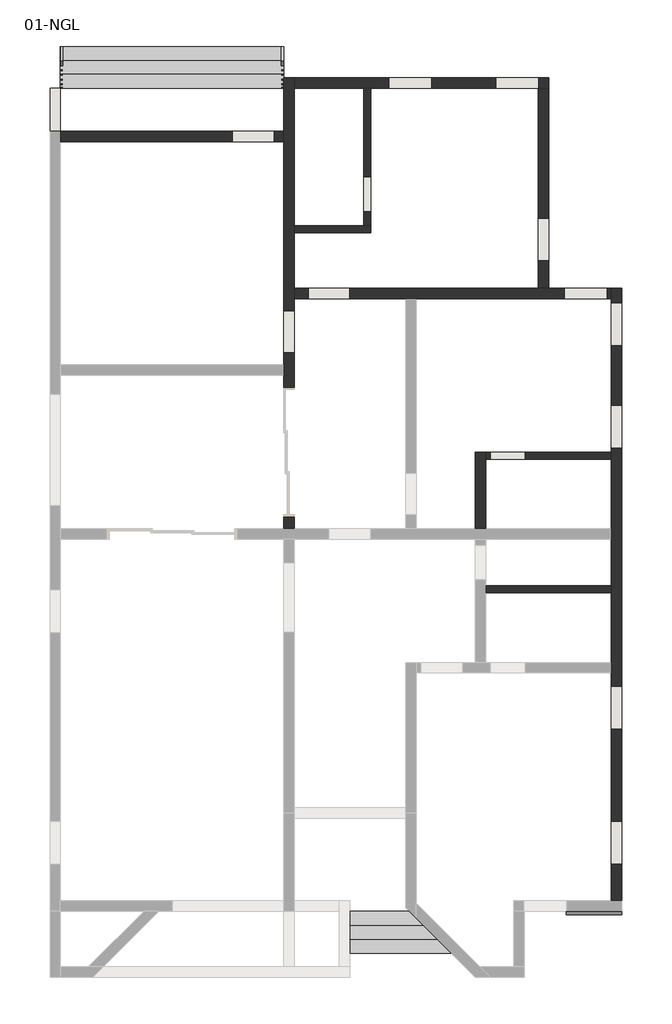
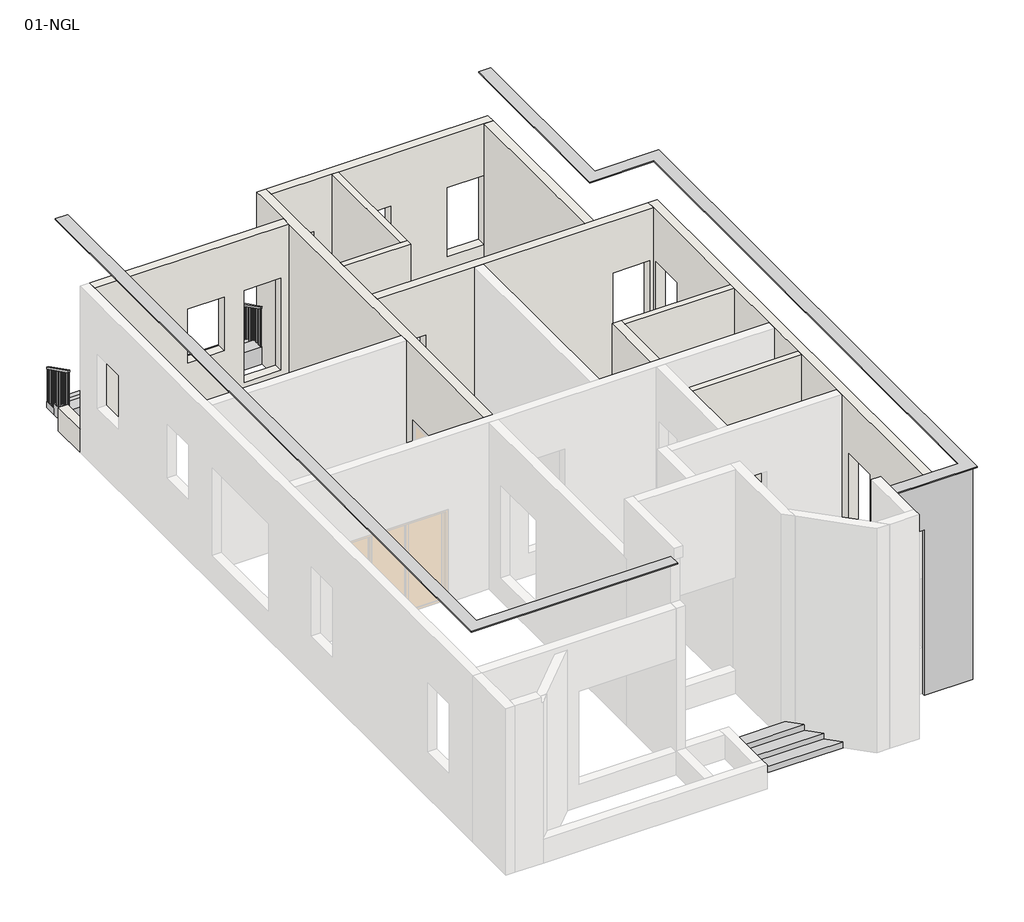
# One storey, part 2 of 2: 12 walls, 2 railings, 2 stair flights, 1 furniture element.
"""IFC4 building model written with IfcOpenShell, lengths in millimetres."""

from ifc_helpers import new_model, si_unit, frame, origin, origin_with_axes, place, context, project, spatial, polyline, outline, extrude, faceted_brep, transform, mapped, element, save
from components import casework_1_casework_1_d55a6497

model = new_model("IFC4")

# Units and contexts
model_context = context("Model", 3, world=origin())
ifc_project = project(units=[si_unit("LENGTHUNIT", "METRE", prefix="MILLI")], contexts=[model_context])

# Site, building, storey
site = spatial("IfcSite", under=ifc_project)
building = spatial("IfcBuilding", under=site)
storey = spatial("IfcBuildingStorey", under=building, Name="01-NGL", Elevation=0.0)

# Furniture
placement = place(None, origin())
casework_1_casework_1_shape = casework_1_casework_1_d55a6497(model_context)
element("IfcFurniture", 1, ObjectType="Casework 1 : Casework 1", at=placement, inside=storey, context=model_context, shape_type="MappedRepresentation", body=[
    mapped(casework_1_casework_1_shape, transform((0.0, 0.0, 0.0), x_axis=(1.0, 0.0, 0.0), y_axis=(0.0, 1.0, 0.0), z_axis=(0.0, 0.0, 1.0))),
])

# Railings
element("IfcRailing", 2, ObjectType="Handrail - Rectangular", at=placement, inside=storey, context=model_context, shape_type="SweptSolid", body=[
    extrude(outline(polyline([(5977.4735, 1050.0), (5977.4735, 994.0983006), (5077.4735, 1444.0983006), (5077.4735, 1500.0), (5977.4735, 1050.0)])), frame((-8660.0564803, 0.0, 0.0), z_axis=(1.0, 0.0, 0.0), x_axis=(0.0, 1.0, 0.0)), (0.0, 0.0, 1.0), 50.0),
    extrude(outline(polyline([(5174.6735, 1395.4983006), (5174.6735, 450.0), (5154.6735, 450.0), (5154.6735, 1405.4983006), (5174.6735, 1395.4983006)])), frame((-8645.0564803, 0.0, 0.0), z_axis=(1.0, 0.0, 0.0), x_axis=(0.0, 1.0, 0.0)), (0.0, 0.0, 1.0), 20.0),
    extrude(outline(polyline([(5276.2735, 1344.6983006), (5276.2735, 450.0), (5256.2735, 450.0), (5256.2735, 1354.6983006), (5276.2735, 1344.6983006)])), frame((-8645.0564803, 0.0, 0.0), z_axis=(1.0, 0.0, 0.0), x_axis=(0.0, 1.0, 0.0)), (0.0, 0.0, 1.0), 20.0),
    extrude(outline(polyline([(5377.8735, 1293.8483006), (5377.8735, 450.0), (5357.8735, 450.0), (5357.8735, 1303.8483006), (5377.8735, 1293.8483006)])), frame((-8645.0564803, 0.0, 0.0), z_axis=(1.0, 0.0, 0.0), x_axis=(0.0, 1.0, 0.0)), (0.0, 0.0, 1.0), 20.0),
    extrude(outline(polyline([(5479.4735, 1243.0983006), (5479.4735, 300.0), (5459.4735, 300.0), (5459.4735, 1253.0983006), (5479.4735, 1243.0983006)])), frame((-8645.0564803, 0.0, 0.0), z_axis=(1.0, 0.0, 0.0), x_axis=(0.0, 1.0, 0.0)), (0.0, 0.0, 1.0), 20.0),
    extrude(outline(polyline([(5581.0735, 1192.2983006), (5581.0735, 300.0), (5561.0735, 300.0), (5561.0735, 1202.2983006), (5581.0735, 1192.2983006)])), frame((-8645.0564803, 0.0, 0.0), z_axis=(1.0, 0.0, 0.0), x_axis=(0.0, 1.0, 0.0)), (0.0, 0.0, 1.0), 20.0),
    extrude(outline(polyline([(5682.6735, 1141.4983006), (5682.6735, 300.0), (5662.6735, 300.0), (5662.6735, 1151.4983006), (5682.6735, 1141.4983006)])), frame((-8645.0564803, 0.0, 0.0), z_axis=(1.0, 0.0, 0.0), x_axis=(0.0, 1.0, 0.0)), (0.0, 0.0, 1.0), 20.0),
    extrude(outline(polyline([(5784.2735, 1090.6983006), (5784.2735, 150.0), (5764.2735, 150.0), (5764.2735, 1100.6983006), (5784.2735, 1090.6983006)])), frame((-8645.0564803, 0.0, 0.0), z_axis=(1.0, 0.0, 0.0), x_axis=(0.0, 1.0, 0.0)), (0.0, 0.0, 1.0), 20.0),
    extrude(outline(polyline([(5885.8735, 1039.8983006), (5885.8735, 150.0), (5865.8735, 150.0), (5865.8735, 1049.8983006), (5885.8735, 1039.8983006)])), frame((-8645.0564803, 0.0, 0.0), z_axis=(1.0, 0.0, 0.0), x_axis=(0.0, 1.0, 0.0)), (0.0, 0.0, 1.0), 20.0),
    extrude(outline(polyline([(5096.9735, 1434.3483006), (5096.9735, 450.0), (5076.9735, 450.0), (5076.9735, 1444.3483006), (5096.9735, 1434.3483006)])), frame((-8645.0564803, 0.0, 0.0), z_axis=(1.0, 0.0, 0.0), x_axis=(0.0, 1.0, 0.0)), (0.0, 0.0, 1.0), 20.0),
    extrude(outline(polyline([(5977.9735, 993.8483006), (5977.9735, 150.0), (5957.9735, 150.0), (5957.9735, 1003.8483006), (5977.9735, 993.8483006)])), frame((-8645.0564803, 0.0, 0.0), z_axis=(1.0, 0.0, 0.0), x_axis=(0.0, 1.0, 0.0)), (0.0, 0.0, 1.0), 20.0),
])
element("IfcRailing", 3, ObjectType="Handrail - Rectangular", at=placement, inside=storey, context=model_context, shape_type="SweptSolid", body=[
    extrude(outline(polyline([(5977.4735, 1050.0), (5977.4735, 994.0983006), (5077.4735, 1444.0983006), (5077.4735, 1500.0), (5977.4735, 1050.0)])), frame((-3910.8564803, 0.0, 0.0), z_axis=(1.0, 0.0, 0.0), x_axis=(0.0, 1.0, 0.0)), (0.0, 0.0, 1.0), 50.0),
    extrude(outline(polyline([(5174.6735, 450.0), (5154.6735, 450.0), (5154.6735, 1405.4983006), (5174.6735, 1395.4983006), (5174.6735, 450.0)])), frame((-3895.8564803, 0.0, 0.0), z_axis=(1.0, 0.0, 0.0), x_axis=(0.0, 1.0, 0.0)), (0.0, 0.0, 1.0), 20.0),
    extrude(outline(polyline([(5276.2735, 450.0), (5256.2735, 450.0), (5256.2735, 1354.6983006), (5276.2735, 1344.6983006), (5276.2735, 450.0)])), frame((-3895.8564803, 0.0, 0.0), z_axis=(1.0, 0.0, 0.0), x_axis=(0.0, 1.0, 0.0)), (0.0, 0.0, 1.0), 20.0),
    extrude(outline(polyline([(5377.8735, 450.0), (5357.8735, 450.0), (5357.8735, 1303.8483006), (5377.8735, 1293.8483006), (5377.8735, 450.0)])), frame((-3895.8564803, 0.0, 0.0), z_axis=(1.0, 0.0, 0.0), x_axis=(0.0, 1.0, 0.0)), (0.0, 0.0, 1.0), 20.0),
    extrude(outline(polyline([(5479.4735, 300.0), (5459.4735, 300.0), (5459.4735, 1253.0983006), (5479.4735, 1243.0983006), (5479.4735, 300.0)])), frame((-3895.8564803, 0.0, 0.0), z_axis=(1.0, 0.0, 0.0), x_axis=(0.0, 1.0, 0.0)), (0.0, 0.0, 1.0), 20.0),
    extrude(outline(polyline([(5581.0735, 300.0), (5561.0735, 300.0), (5561.0735, 1202.2983006), (5581.0735, 1192.2983006), (5581.0735, 300.0)])), frame((-3895.8564803, 0.0, 0.0), z_axis=(1.0, 0.0, 0.0), x_axis=(0.0, 1.0, 0.0)), (0.0, 0.0, 1.0), 20.0),
    extrude(outline(polyline([(5682.6735, 300.0), (5662.6735, 300.0), (5662.6735, 1151.4983006), (5682.6735, 1141.4983006), (5682.6735, 300.0)])), frame((-3895.8564803, 0.0, 0.0), z_axis=(1.0, 0.0, 0.0), x_axis=(0.0, 1.0, 0.0)), (0.0, 0.0, 1.0), 20.0),
    extrude(outline(polyline([(5784.2735, 150.0), (5764.2735, 150.0), (5764.2735, 1100.6983006), (5784.2735, 1090.6983006), (5784.2735, 150.0)])), frame((-3895.8564803, 0.0, 0.0), z_axis=(1.0, 0.0, 0.0), x_axis=(0.0, 1.0, 0.0)), (0.0, 0.0, 1.0), 20.0),
    extrude(outline(polyline([(5885.8735, 150.0), (5865.8735, 150.0), (5865.8735, 1049.8983006), (5885.8735, 1039.8983006), (5885.8735, 150.0)])), frame((-3895.8564803, 0.0, 0.0), z_axis=(1.0, 0.0, 0.0), x_axis=(0.0, 1.0, 0.0)), (0.0, 0.0, 1.0), 20.0),
    extrude(outline(polyline([(5096.9735, 450.0), (5076.9735, 450.0), (5076.9735, 1444.3483006), (5096.9735, 1434.3483006), (5096.9735, 450.0)])), frame((-3895.8564803, 0.0, 0.0), z_axis=(1.0, 0.0, 0.0), x_axis=(0.0, 1.0, 0.0)), (0.0, 0.0, 1.0), 20.0),
    extrude(outline(polyline([(5977.9735, 150.0), (5957.9735, 150.0), (5957.9735, 1003.8483006), (5977.9735, 993.8483006), (5977.9735, 150.0)])), frame((-3895.8564803, 0.0, 0.0), z_axis=(1.0, 0.0, 0.0), x_axis=(0.0, 1.0, 0.0)), (0.0, 0.0, 1.0), 20.0),
])

# Stair flights
element("IfcStairFlight", 4, at=placement, inside=storey, context=model_context, shape_type="Brep", body=[
    faceted_brep([(-2435.4564803, -13222.5265, 150.0), (-2435.4564803, -13522.5265, 150.0), (-260.4564803, -13522.5265, 150.0), (-560.4564803, -13222.5265, 150.0), (-2435.4564803, -13222.5265, 0.0), (-2435.4564803, -13522.5265, 0.0), (-260.4564803, -13522.5265, 0.0), (-560.4564803, -13222.5265, 0.0), (-2435.4564803, -12922.5265, 300.0), (-2435.4564803, -13222.5265, 300.0), (-560.4564803, -13222.5265, 300.0), (-860.4564803, -12922.5265, 300.0), (-2435.4564803, -12922.5265, 0.0), (-860.4564803, -12922.5265, 0.0), (-2435.4564803, -12622.5265, 450.0), (-2435.4564803, -12922.5265, 450.0), (-860.4564803, -12922.5265, 450.0), (-1160.4564803, -12622.5265, 450.0), (-2435.4564803, -12622.5265, 0.0), (-1160.4564803, -12622.5265, 0.0)], [[[0, 1, 2, 3]], [[1, 0, 4, 5]], [[2, 1, 5, 6]], [[3, 2, 6, 7]], [[8, 9, 10, 11]], [[4, 0, 9, 8, 12]], [[0, 3, 10, 9]], [[3, 7, 13, 11, 10]], [[14, 15, 16, 17]], [[12, 8, 15, 14, 18]], [[8, 11, 16, 15]], [[11, 13, 19, 17, 16]], [[14, 17, 19, 18]], [[5, 4, 12, 18, 19, 13, 7, 6]]]),
])
element("IfcStairFlight", 5, at=placement, inside=storey, context=model_context, shape_type="Brep", body=[
    faceted_brep([(-3860.4564803, 5677.4735, 150.0), (-3860.4564803, 5977.4735, 150.0), (-8660.4564803, 5977.4735, 150.0), (-8660.4564803, 5677.4735, 150.0), (-3860.4564803, 5677.4735, 0.0), (-3860.4564803, 5977.4735, 0.0), (-8660.4564803, 5977.4735, 0.0), (-8660.4564803, 5677.4735, 0.0), (-3860.4564803, 5377.4735, 300.0), (-3860.4564803, 5677.4735, 300.0), (-8660.4564803, 5677.4735, 300.0), (-8660.4564803, 5377.4735, 300.0), (-3860.4564803, 5377.4735, 0.0), (-8660.4564803, 5377.4735, 0.0), (-3860.4564803, 5077.4735, 450.0), (-3860.4564803, 5377.4735, 450.0), (-8660.4564803, 5377.4735, 450.0), (-8660.4564803, 5077.4735, 450.0), (-3860.4564803, 5077.4735, 0.0), (-8660.4564803, 5077.4735, 0.0)], [[[0, 1, 2, 3]], [[1, 0, 4, 5]], [[2, 1, 5, 6]], [[3, 2, 6, 7]], [[8, 9, 10, 11]], [[4, 0, 9, 8, 12]], [[0, 3, 10, 9]], [[3, 7, 13, 11, 10]], [[14, 15, 16, 17]], [[12, 8, 15, 14, 18]], [[8, 11, 16, 15]], [[11, 13, 19, 17, 16]], [[14, 17, 19, 18]], [[5, 4, 12, 18, 19, 13, 7, 6]]]),
])

# Walls
element("IfcWall", 6, ObjectType="01-225 wall", at=placement, inside=storey, context=model_context, shape_type="Brep", body=[
    faceted_brep([(3414.5435197, -12397.5265, 0.0), (3414.5435197, 777.4735, 0.0), (3414.5435197, 777.4735, 4350.0), (3414.5435197, -12397.5265, 4350.0), (3414.5435197, -10697.5265, 3000.0), (3414.5435197, -10697.5265, 1200.0), (3414.5435197, -11597.5265, 1200.0), (3414.5435197, -11597.5265, 3000.0), (3414.5435197, -8697.5265, 3000.0), (3414.5435197, -7797.5265, 3000.0), (3414.5435197, -7797.5265, 1200.0), (3414.5435197, -8697.5265, 1200.0), (3414.5435197, -1747.5265, 3000.0), (3414.5435197, -1747.5265, 1200.0), (3414.5435197, -2647.5265, 1200.0), (3414.5435197, -2647.5265, 3000.0), (3414.5435197, 452.4735, 3000.0), (3414.5435197, 452.4735, 1200.0), (3414.5435197, -447.5265, 1200.0), (3414.5435197, -447.5265, 3000.0), (3414.5435197, -6822.5265, 3000.0), (3414.5435197, -6222.5265, 3000.0), (3414.5435197, -6222.5265, 1800.0), (3414.5435197, -6822.5265, 1800.0), (3414.5435197, -3347.5265, 3000.0), (3414.5435197, -3347.5265, 1800.0), (3414.5435197, -3947.5265, 1800.0), (3414.5435197, -3947.5265, 3000.0), (3189.5435197, -12397.5265, 0.0), (3189.5435197, -12397.5265, 4350.0), (3189.5435197, -7497.5265, 4350.0), (3189.5435197, -7272.5265, 4350.0), (3189.5435197, -5772.5265, 4350.0), (3189.5435197, -5622.5265, 4350.0), (3189.5435197, -4622.5265, 4350.0), (3189.5435197, -4397.5265, 4350.0), (3189.5435197, -2897.5265, 4350.0), (3189.5435197, -2747.5265, 4350.0), (3189.5435197, 552.4735, 4350.0), (3189.5435197, 777.4735, 4350.0), (3189.5435197, 777.4735, 0.0), (3189.5435197, 552.4735, 0.0), (3189.5435197, -2747.5265, 0.0), (3189.5435197, -2897.5265, 0.0), (3189.5435197, -4397.5265, 0.0), (3189.5435197, -4622.5265, 0.0), (3189.5435197, -5622.5265, 0.0), (3189.5435197, -5772.5265, 0.0), (3189.5435197, -7272.5265, 0.0), (3189.5435197, -7497.5265, 0.0), (3189.5435197, -10697.5265, 3000.0), (3189.5435197, -11597.5265, 3000.0), (3189.5435197, -11597.5265, 1200.0), (3189.5435197, -10697.5265, 1200.0), (3189.5435197, -8697.5265, 3000.0), (3189.5435197, -8697.5265, 1200.0), (3189.5435197, -7797.5265, 1200.0), (3189.5435197, -7797.5265, 3000.0), (3189.5435197, -1747.5265, 3000.0), (3189.5435197, -2647.5265, 3000.0), (3189.5435197, -2647.5265, 1200.0), (3189.5435197, -1747.5265, 1200.0), (3189.5435197, 452.4735, 3000.0), (3189.5435197, -447.5265, 3000.0), (3189.5435197, -447.5265, 1200.0), (3189.5435197, 452.4735, 1200.0), (3189.5435197, -6822.5265, 3000.0), (3189.5435197, -6822.5265, 1800.0), (3189.5435197, -6222.5265, 1800.0), (3189.5435197, -6222.5265, 3000.0), (3189.5435197, -3347.5265, 3000.0), (3189.5435197, -3947.5265, 3000.0), (3189.5435197, -3947.5265, 1800.0), (3189.5435197, -3347.5265, 1800.0)], [[[0, 1, 2, 3], [4, 5, 6, 7], [8, 9, 10, 11], [12, 13, 14, 15], [16, 17, 18, 19], [20, 21, 22, 23], [24, 25, 26, 27]], [[28, 29, 30, 31, 32, 33, 34, 35, 36, 37, 38, 39, 40, 41, 42, 43, 44, 45, 46, 47, 48, 49], [50, 51, 52, 53], [54, 55, 56, 57], [58, 59, 60, 61], [62, 63, 64, 65], [66, 67, 68, 69], [70, 71, 72, 73]], [[1, 0, 28, 49, 48, 47, 46, 45, 44, 43, 42, 41, 40]], [[3, 2, 39, 38, 37, 36, 35, 34, 33, 32, 31, 30, 29]], [[0, 3, 29, 28]], [[2, 1, 40, 39]], [[5, 4, 50, 53]], [[6, 5, 53, 52]], [[7, 6, 52, 51]], [[4, 7, 51, 50]], [[55, 54, 8, 11]], [[56, 55, 11, 10]], [[57, 56, 10, 9]], [[54, 57, 9, 8]], [[13, 12, 58, 61]], [[14, 13, 61, 60]], [[15, 14, 60, 59]], [[12, 15, 59, 58]], [[17, 16, 62, 65]], [[18, 17, 65, 64]], [[19, 18, 64, 63]], [[16, 19, 63, 62]], [[67, 66, 20, 23]], [[68, 67, 23, 22]], [[69, 68, 22, 21]], [[66, 69, 21, 20]], [[25, 24, 70, 73]], [[26, 25, 73, 72]], [[27, 26, 72, 71]], [[24, 27, 71, 70]]]),
])
element("IfcWall", 7, ObjectType="01-225 wall", at=placement, inside=storey, context=model_context, shape_type="Brep", body=[
    faceted_brep([(3189.5435197, 777.4735, 0.0), (1839.5435197, 777.4735, 0.0), (1614.5435197, 777.4735, 0.0), (-3635.4564803, 777.4735, 0.0), (-3635.4564803, 777.4735, 4350.0), (1614.5435197, 777.4735, 4350.0), (1839.5435197, 777.4735, 4350.0), (3189.5435197, 777.4735, 4350.0), (-3335.4564803, 777.4735, 600.0), (-2435.4564803, 777.4735, 600.0), (-2435.4564803, 777.4735, 3000.0), (-3335.4564803, 777.4735, 3000.0), (2189.5435197, 777.4735, 3000.0), (2189.5435197, 777.4735, 1200.0), (3089.5435197, 777.4735, 1200.0), (3089.5435197, 777.4735, 3000.0), (3189.5435197, 552.4735, 0.0), (3189.5435197, 552.4735, 4350.0), (-1010.4564803, 552.4735, 4350.0), (-1235.4564803, 552.4735, 4350.0), (-3635.4564803, 552.4735, 4350.0), (-3635.4564803, 552.4735, 0.0), (-1235.4564803, 552.4735, 0.0), (-1010.4564803, 552.4735, 0.0), (-3335.4564803, 552.4735, 600.0), (-3335.4564803, 552.4735, 3000.0), (-2435.4564803, 552.4735, 3000.0), (-2435.4564803, 552.4735, 600.0), (2189.5435197, 552.4735, 3000.0), (3089.5435197, 552.4735, 3000.0), (3089.5435197, 552.4735, 1200.0), (2189.5435197, 552.4735, 1200.0)], [[[0, 1, 2, 3, 4, 5, 6, 7], [8, 9, 10, 11], [12, 13, 14, 15]], [[16, 17, 18, 19, 20, 21, 22, 23], [24, 25, 26, 27], [28, 29, 30, 31]], [[3, 2, 1, 0, 16, 23, 22, 21]], [[7, 6, 5, 4, 20, 19, 18, 17]], [[0, 7, 17, 16]], [[4, 3, 21, 20]], [[25, 24, 8, 11]], [[26, 25, 11, 10]], [[27, 26, 10, 9]], [[24, 27, 9, 8]], [[13, 12, 28, 31]], [[14, 13, 31, 30]], [[15, 14, 30, 29]], [[12, 15, 29, 28]]]),
])
element("IfcWall", 8, ObjectType="01-225 wall", at=placement, inside=storey, context=model_context, shape_type="SweptSolid", body=[
    extrude(outline(polyline([(4350.0, -8660.4564803), (0.0, -8660.4564803), (0.0, -3860.4564803), (4350.0, -3860.4564803), (4350.0, -8660.4564803)]), holes=[polyline([(600.0, -4060.4564803), (600.0, -4960.4564803), (3000.0, -4960.4564803), (3000.0, -4060.4564803), (600.0, -4060.4564803)]), polyline([(3000.0, -5460.4564803), (1600.0, -5460.4564803), (1600.0, -6360.4564803), (3000.0, -6360.4564803), (3000.0, -5460.4564803)])]), frame((0.0, 3927.4735, 0.0), z_axis=(0.0, 1.0, 0.0), x_axis=(0.0, 0.0, 1.0)), (0.0, 0.0, 1.0), 225.0),
])
element("IfcWall", 9, ObjectType="01-225 wall", at=placement, inside=storey, context=model_context, shape_type="Brep", body=[
    faceted_brep([(-3635.4564803, 5302.4735, 4350.0), (-3635.4564803, 5077.4735, 4350.0), (-3635.4564803, 2127.4735, 4350.0), (-3635.4564803, 1977.4735, 4350.0), (-3635.4564803, 777.4735, 4350.0), (-3635.4564803, 552.4735, 4350.0), (-3635.4564803, -4397.5265, 4350.0), (-3635.4564803, -4397.5265, 0.0), (-3635.4564803, -4137.5265, 0.0), (-3635.4564803, -4137.5265, 2440.0), (-3635.4564803, -1357.5265, 2440.0), (-3635.4564803, -1357.5265, 0.0), (-3635.4564803, 552.4735, 0.0), (-3635.4564803, 777.4735, 0.0), (-3635.4564803, 1977.4735, 0.0), (-3635.4564803, 2127.4735, 0.0), (-3635.4564803, 5077.4735, 0.0), (-3635.4564803, 5302.4735, 0.0), (-3635.4564803, -610.0265, 600.0), (-3635.4564803, -610.0265, 3000.0), (-3635.4564803, 289.9735, 3000.0), (-3635.4564803, 289.9735, 600.0), (-3860.4564803, -4397.5265, 4350.0), (-3860.4564803, -1097.5265, 4350.0), (-3860.4564803, -872.5265, 4350.0), (-3860.4564803, 3927.4735, 4350.0), (-3860.4564803, 4152.4735, 4350.0), (-3860.4564803, 5077.4735, 4350.0), (-3860.4564803, 5302.4735, 4350.0), (-3860.4564803, 5302.4735, 3900.0), (-3860.4564803, 5302.4735, 0.0), (-3860.4564803, 4152.4735, 0.0), (-3860.4564803, 3927.4735, 0.0), (-3860.4564803, -872.5265, 0.0), (-3860.4564803, -1097.5265, 0.0), (-3860.4564803, -1357.5265, 0.0), (-3860.4564803, -1357.5265, 2440.0), (-3860.4564803, -4137.5265, 2440.0), (-3860.4564803, -4137.5265, 0.0), (-3860.4564803, -4397.5265, 0.0), (-3860.4564803, -610.0265, 600.0), (-3860.4564803, 289.9735, 600.0), (-3860.4564803, 289.9735, 3000.0), (-3860.4564803, -610.0265, 3000.0)], [[[0, 1, 2, 3, 4, 5, 6, 7, 8, 9, 10, 11, 12, 13, 14, 15, 16, 17], [18, 19, 20, 21]], [[22, 23, 24, 25, 26, 27, 28, 29, 30, 31, 32, 33, 34, 35, 36, 37, 38, 39], [40, 41, 42, 43]], [[30, 17, 16, 15, 14, 13, 12, 11, 35, 34, 33, 32, 31]], [[7, 39, 38, 8]], [[6, 5, 4, 3, 2, 1, 0, 28, 27, 26, 25, 24, 23, 22]], [[7, 6, 22, 39]], [[19, 18, 40, 43]], [[20, 19, 43, 42]], [[21, 20, 42, 41]], [[18, 21, 41, 40]], [[10, 36, 35, 11]], [[36, 10, 9, 37]], [[37, 9, 8, 38]], [[17, 30, 29, 28, 0]]]),
])
element("IfcWall", 10, ObjectType="01-225 wall", at=placement, inside=storey, context=model_context, shape_type="Brep", body=[
    faceted_brep([(-3635.4564803, 5077.4735, 4350.0), (-3635.4564803, 5077.4735, 0.0), (-2135.4564803, 5077.4735, 0.0), (-1985.4564803, 5077.4735, 0.0), (1614.5435197, 5077.4735, 0.0), (1839.5435197, 5077.4735, 0.0), (1839.5435197, 5077.4735, 4350.0), (1614.5435197, 5077.4735, 4350.0), (-1985.4564803, 5077.4735, 4350.0), (-2135.4564803, 5077.4735, 4350.0), (1614.5435197, 5077.4735, 3000.0), (1614.5435197, 5077.4735, 1200.0), (714.5435197, 5077.4735, 1200.0), (714.5435197, 5077.4735, 3000.0), (-685.4564803, 5077.4735, 3000.0), (-685.4564803, 5077.4735, 1200.0), (-1585.4564803, 5077.4735, 1200.0), (-1585.4564803, 5077.4735, 3000.0), (-2585.4564803, 5077.4735, 3000.0), (-2585.4564803, 5077.4735, 1800.0), (-3185.4564803, 5077.4735, 1800.0), (-3185.4564803, 5077.4735, 3000.0), (-3635.4564803, 5302.4735, 0.0), (-3635.4564803, 5302.4735, 4350.0), (1839.5435197, 5302.4735, 4350.0), (1839.5435197, 5302.4735, 0.0), (1614.5435197, 5302.4735, 3000.0), (714.5435197, 5302.4735, 3000.0), (714.5435197, 5302.4735, 1200.0), (1614.5435197, 5302.4735, 1200.0), (-685.4564803, 5302.4735, 3000.0), (-1585.4564803, 5302.4735, 3000.0), (-1585.4564803, 5302.4735, 1200.0), (-685.4564803, 5302.4735, 1200.0), (-2585.4564803, 5302.4735, 3000.0), (-3185.4564803, 5302.4735, 3000.0), (-3185.4564803, 5302.4735, 1800.0), (-2585.4564803, 5302.4735, 1800.0)], [[[0, 1, 2, 3, 4, 5, 6, 7, 8, 9], [10, 11, 12, 13], [14, 15, 16, 17], [18, 19, 20, 21]], [[22, 23, 24, 25], [26, 27, 28, 29], [30, 31, 32, 33], [34, 35, 36, 37]], [[5, 4, 3, 2, 1, 22, 25]], [[0, 9, 8, 7, 6, 24, 23]], [[6, 5, 25, 24]], [[11, 10, 26, 29]], [[12, 11, 29, 28]], [[13, 12, 28, 27]], [[10, 13, 27, 26]], [[15, 14, 30, 33]], [[16, 15, 33, 32]], [[17, 16, 32, 31]], [[14, 17, 31, 30]], [[19, 18, 34, 37]], [[20, 19, 37, 36]], [[21, 20, 36, 35]], [[18, 21, 35, 34]], [[0, 23, 22, 1]]]),
])
element("IfcWall", 11, ObjectType="01-225 wall", at=placement, inside=storey, context=model_context, shape_type="Brep", body=[
    faceted_brep([(1614.5435197, 5077.4735, 0.0), (1614.5435197, 777.4735, 0.0), (1614.5435197, 777.4735, 4350.0), (1614.5435197, 5077.4735, 4350.0), (1614.5435197, 5077.4735, 3000.0), (1614.5435197, 5077.4735, 1200.0), (1614.5435197, 1377.4735, 3000.0), (1614.5435197, 1377.4735, 1200.0), (1614.5435197, 2277.4735, 1200.0), (1614.5435197, 2277.4735, 3000.0), (1839.5435197, 5077.4735, 0.0), (1839.5435197, 5077.4735, 4350.0), (1839.5435197, 777.4735, 4350.0), (1839.5435197, 777.4735, 0.0), (1839.5435197, 1377.4735, 3000.0), (1839.5435197, 2277.4735, 3000.0), (1839.5435197, 2277.4735, 1200.0), (1839.5435197, 1377.4735, 1200.0)], [[[0, 1, 2, 3, 4, 5], [6, 7, 8, 9]], [[10, 11, 12, 13], [14, 15, 16, 17]], [[1, 0, 10, 13]], [[3, 2, 12, 11]], [[0, 5, 4, 3, 11, 10]], [[2, 1, 13, 12]], [[7, 6, 14, 17]], [[8, 7, 17, 16]], [[9, 8, 16, 15]], [[6, 9, 15, 14]]]),
])
element("IfcWall", 12, ObjectType="01-225 wall", at=placement, inside=storey, context=model_context, shape_type="Brep", body=[
    faceted_brep([(489.5435197, -4397.5265, 0.0), (489.5435197, -2897.5265, 0.0), (489.5435197, -2747.5265, 0.0), (489.5435197, -2747.5265, 4350.0), (489.5435197, -2897.5265, 4350.0), (489.5435197, -4397.5265, 4350.0), (264.5435197, -4397.5265, 0.0), (264.5435197, -4397.5265, 4350.0), (264.5435197, -2747.5265, 4350.0), (264.5435197, -2747.5265, 0.0)], [[[0, 1, 2, 3, 4, 5]], [[6, 7, 8, 9]], [[2, 1, 0, 6, 9]], [[5, 4, 3, 8, 7]], [[0, 5, 7, 6]], [[3, 2, 9, 8]]]),
])
element("IfcWall", 13, ObjectType="01-225 wall", at=placement, inside=storey, context=model_context, shape_type="SweptSolid", body=[
    extrude(outline(polyline([(-8660.4564803, 5077.4735), (-8660.4564803, 4152.4735), (-8885.4564803, 4152.4735), (-8885.4564803, 5077.4735), (-8660.4564803, 5077.4735)])), origin_with_axes(), (0.0, 0.0, 1.0), 625.0),
])
element("IfcWall", 14, ObjectType="02-150 WALL", at=placement, inside=storey, context=model_context, shape_type="SweptSolid", body=[
    extrude(outline(polyline([(3189.5435197, -5772.5265), (489.5435197, -5772.5265), (489.5435197, -5622.5265), (3189.5435197, -5622.5265), (3189.5435197, -5772.5265)])), origin_with_axes(), (0.0, 0.0, 1.0), 4350.0),
])
element("IfcWall", 15, ObjectType="02-150 WALL", at=placement, inside=storey, context=model_context, shape_type="SweptSolid", body=[
    extrude(outline(polyline([(0.0, 489.5435197), (0.0, 3189.5435197), (4350.0, 3189.5435197), (4350.0, 489.5435197), (0.0, 489.5435197)]), holes=[polyline([(600.0, 589.5435197), (3000.0, 589.5435197), (3000.0, 1339.5435197), (600.0, 1339.5435197), (600.0, 589.5435197)])]), frame((0.0, -2897.5265, 0.0), z_axis=(0.0, 1.0, 0.0), x_axis=(0.0, 0.0, 1.0)), (0.0, 0.0, 1.0), 150.0),
])
element("IfcWall", 16, ObjectType="02-150 WALL", at=placement, inside=storey, context=model_context, shape_type="Brep", body=[
    faceted_brep([(-3635.4564803, 1977.4735, 0.0), (-1985.4564803, 1977.4735, 0.0), (-1985.4564803, 1977.4735, 4350.0), (-3635.4564803, 1977.4735, 4350.0), (-3635.4564803, 2127.4735, 0.0), (-3635.4564803, 2127.4735, 4350.0), (-2135.4564803, 2127.4735, 4350.0), (-1985.4564803, 2127.4735, 4350.0), (-1985.4564803, 2127.4735, 0.0), (-2135.4564803, 2127.4735, 0.0)], [[[0, 1, 2, 3]], [[4, 5, 6, 7, 8, 9]], [[1, 0, 4, 9, 8]], [[3, 2, 7, 6, 5]], [[0, 3, 5, 4]], [[2, 1, 8, 7]]]),
])
element("IfcWall", 17, ObjectType="02-150 WALL", at=placement, inside=storey, context=model_context, shape_type="SweptSolid", body=[
    extrude(outline(polyline([(2127.4735, 0.0), (2127.4735, 4350.0), (5077.4735, 4350.0), (5077.4735, 0.0), (2127.4735, 0.0)]), holes=[polyline([(2427.4735, 600.0), (3177.4735, 600.0), (3177.4735, 3000.0), (2427.4735, 3000.0), (2427.4735, 600.0)])]), frame((-2135.4564803, 0.0, 0.0), z_axis=(1.0, 0.0, 0.0), x_axis=(0.0, 1.0, 0.0)), (0.0, 0.0, 1.0), 150.0),
])

save(model, "model.ifc")

# Revit data of these elements
# Type "Handrail - Rectangular"
#   Assembly Code = "C2010400"
#   built-in parameter 1008612 = 0.0416667 (stored number, unit not read)
#   built-in parameter 1008611 = 0.0416667 (stored number, unit not read)
#   built-in parameter 1008609 = 0.333333 (stored number, unit not read)
#   built-in parameter 1008604 = 0.166667 (stored number, unit not read)
#   built-in parameter 1008603 = 0.166667 (stored number, unit not read)
#   Railing Height = 900 mm
#   built-in parameter 1008630 = 2
#   built-in parameter 1008610 = 2
# Type "01-225 wall"
#   Description = "Generic Wall (Material By Category), 200mm thick"
#   Assembly Code = "B2010"
#   Type Mark = "G06"
#   Layers, outside or top first: 225 mm "01-225 wall paint" (function 1)
# Type "02-150 WALL"
#   Description = "Generic Wall (Material By Category), 200mm thick"
#   Assembly Code = "B2010"
#   Type Mark = "G06"
#   Layers, outside or top first: 150 mm "01-225 wall paint" (function 1)
# Element 1 (IfcFurniture, "Casework 1 : Casework 1")
#   Phase Created = New Construction
# Elements 2, 3 (IfcRailing, "Handrail - Rectangular")
#   Phase Created = New Construction
# Elements 4, 5 (IfcStairFlight)
#   Phase Created = New Construction
#   Materials on its faces: "st"
# Elements 6, 7, 8, 9, 10, 11, 12 (IfcWall, "01-225 wall")
#   Top Offset = 0 mm
#   Base Offset = 0 mm
#   wall height = 4350 mm
#   Phase Created = New Construction
#   Base Constraint = 01-NGL
#   Top Constraint = 05-ROOF
#   Materials on its faces: "01-225 wall paint"
# Element 13 (IfcWall, "01-225 wall")
#   Top Offset = 25 mm
#   Base Offset = 0 mm
#   wall height = 625 mm
#   Phase Created = New Construction
#   Base Constraint = 01-NGL
#   Top Constraint = 02-DPC
#   Materials on its faces: "01-225 wall paint"
# Elements 14, 15, 16, 17 (IfcWall, "02-150 WALL")
#   Top Offset = 0 mm
#   Base Offset = 0 mm
#   wall height = 4350 mm
#   Phase Created = New Construction
#   Base Constraint = 01-NGL
#   Top Constraint = 05-ROOF
#   Materials on its faces: "01-225 wall paint"
# Materials
#   "01-225 wall paint": class "Generic", colour RGB 242 242 255, transparency 0, Cost = 0
#   "st": class "Generic", colour RGB 153 149 149, transparency 0, Cost = 0
